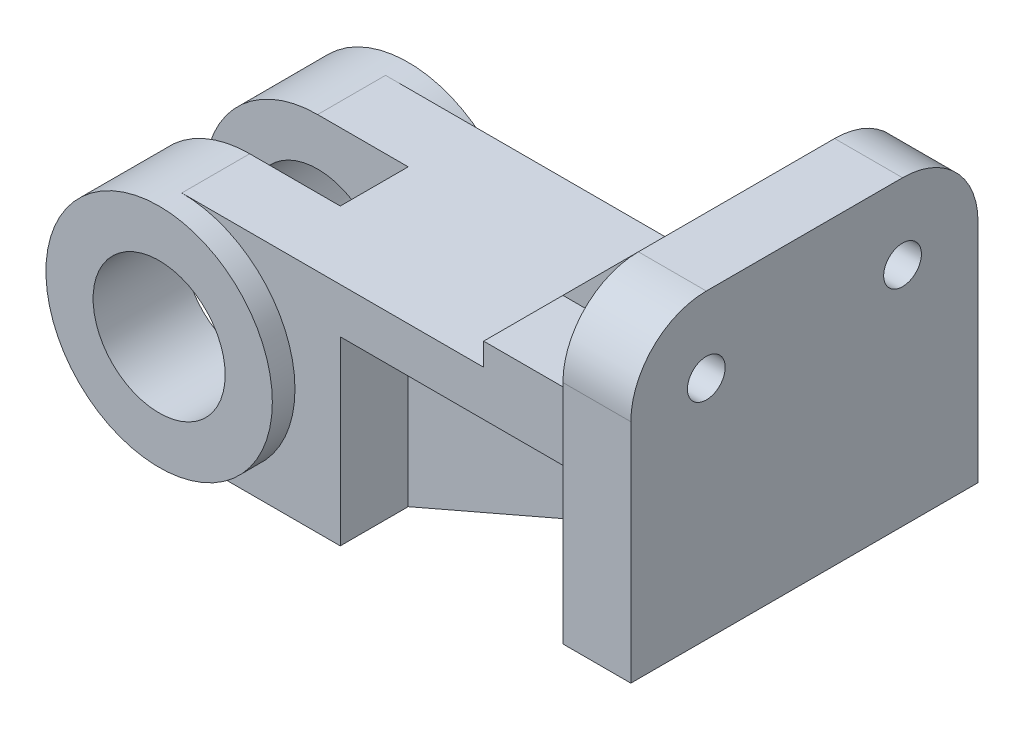
ISO-10303-21;
HEADER;
FILE_DESCRIPTION(('STEP AP214'),'2;1');
FILE_NAME('part.step','',(''),(''),'','','');
FILE_SCHEMA(('AUTOMOTIVE_DESIGN { 1 0 10303 214 1 1 1 1 }'));
ENDSEC;
DATA;
#1=APPLICATION_CONTEXT('core data for automotive mechanical design processes');
#2=APPLICATION_PROTOCOL_DEFINITION('international standard','automotive_design',2000,#1);
#3=PRODUCT_CONTEXT('',#1,'mechanical');
#4=PRODUCT('Part','Part','',(#3));
#5=PRODUCT_RELATED_PRODUCT_CATEGORY('part','',(#4));
#6=PRODUCT_DEFINITION_FORMATION('','',#4);
#7=PRODUCT_DEFINITION_CONTEXT('part definition',#1,'design');
#8=PRODUCT_DEFINITION('design','',#6,#7);
#9=PRODUCT_DEFINITION_SHAPE('','',#8);
#10=(LENGTH_UNIT() NAMED_UNIT(*) SI_UNIT(.MILLI.,.METRE.));
#11=(NAMED_UNIT(*) PLANE_ANGLE_UNIT() SI_UNIT($,.RADIAN.));
#12=(NAMED_UNIT(*) SI_UNIT($,.STERADIAN.) SOLID_ANGLE_UNIT());
#13=UNCERTAINTY_MEASURE_WITH_UNIT(LENGTH_MEASURE(1.E-05),#10,'distance_accuracy_value','');
#14=(GEOMETRIC_REPRESENTATION_CONTEXT(3) GLOBAL_UNCERTAINTY_ASSIGNED_CONTEXT((#13)) GLOBAL_UNIT_ASSIGNED_CONTEXT((#10,
#11,#12)) REPRESENTATION_CONTEXT('',''));
#15=CARTESIAN_POINT('',(0.,0.,0.));
#16=DIRECTION('',(0.,0.,1.));
#17=DIRECTION('',(1.,0.,0.));
#18=AXIS2_PLACEMENT_3D('',#15,#16,#17);
#19=CARTESIAN_POINT('',(0.,0.,33.));
#20=DIRECTION('',(0.,0.,-1.));
#21=DIRECTION('',(-1.,0.,0.));
#22=AXIS2_PLACEMENT_3D('',#19,#20,#21);
#23=CYLINDRICAL_SURFACE('',#22,30.);
#24=CARTESIAN_POINT('',(0.,0.,-33.));
#25=DIRECTION('',(0.,0.,1.));
#26=DIRECTION('',(1.,0.,0.));
#27=AXIS2_PLACEMENT_3D('',#24,#25,#26);
#28=CIRCLE('',#27,30.);
#29=CARTESIAN_POINT('',(30.,0.,-33.));
#30=VERTEX_POINT('',#29);
#31=EDGE_CURVE('E454',#30,#30,#28,.T.);
#32=ORIENTED_EDGE('',*,*,#31,.T.);
#33=EDGE_LOOP('',(#32));
#34=FACE_BOUND('',#33,.T.);
#35=DIRECTION('',(0.,0.,-1.));
#36=VECTOR('',#35,1.);
#37=CARTESIAN_POINT('',(0.,-30.,27.));
#38=LINE('',#37,#36);
#39=CARTESIAN_POINT('',(0.,-30.,-9.));
#40=VERTEX_POINT('',#39);
#41=CARTESIAN_POINT('',(0.,-30.,-27.));
#42=VERTEX_POINT('',#41);
#43=EDGE_CURVE('E446',#40,#42,#38,.T.);
#44=ORIENTED_EDGE('',*,*,#43,.F.);
#45=CARTESIAN_POINT('',(0.,0.,-9.));
#46=DIRECTION('',(0.,0.,-1.));
#47=DIRECTION('',(-1.,0.,0.));
#48=AXIS2_PLACEMENT_3D('',#45,#46,#47);
#49=CIRCLE('',#48,30.);
#50=CARTESIAN_POINT('',(0.,30.,-9.));
#51=VERTEX_POINT('',#50);
#52=EDGE_CURVE('E256',#40,#51,#49,.T.);
#53=ORIENTED_EDGE('',*,*,#52,.T.);
#54=DIRECTION('',(0.,0.,-1.));
#55=VECTOR('',#54,1.);
#56=CARTESIAN_POINT('',(0.,30.,27.));
#57=LINE('',#56,#55);
#58=CARTESIAN_POINT('',(0.,30.,-27.));
#59=VERTEX_POINT('',#58);
#60=EDGE_CURVE('E388',#51,#59,#57,.T.);
#61=ORIENTED_EDGE('',*,*,#60,.T.);
#62=CARTESIAN_POINT('',(0.,0.,-27.));
#63=DIRECTION('',(0.,0.,-1.));
#64=DIRECTION('',(1.,0.,0.));
#65=AXIS2_PLACEMENT_3D('',#62,#63,#64);
#66=CIRCLE('',#65,30.);
#67=EDGE_CURVE('E365',#59,#42,#66,.T.);
#68=ORIENTED_EDGE('',*,*,#67,.T.);
#69=EDGE_LOOP('',(#44,#53,#61,#68));
#70=FACE_BOUND('',#69,.T.);
#71=ADVANCED_FACE('F44',(#34,#70),#23,.T.);
#72=CARTESIAN_POINT('',(0.,0.,33.));
#73=DIRECTION('',(0.,0.,-1.));
#74=DIRECTION('',(-1.,0.,0.));
#75=AXIS2_PLACEMENT_3D('',#72,#73,#74);
#76=CYLINDRICAL_SURFACE('',#75,17.5);
#77=CARTESIAN_POINT('',(0.,0.,-9.));
#78=DIRECTION('',(0.,0.,-1.));
#79=DIRECTION('',(-1.,0.,0.));
#80=AXIS2_PLACEMENT_3D('',#77,#78,#79);
#81=CIRCLE('',#80,17.5);
#82=CARTESIAN_POINT('',(-17.5,0.,-9.));
#83=VERTEX_POINT('',#82);
#84=EDGE_CURVE('E254',#83,#83,#81,.T.);
#85=ORIENTED_EDGE('',*,*,#84,.F.);
#86=EDGE_LOOP('',(#85));
#87=FACE_BOUND('',#86,.T.);
#88=CARTESIAN_POINT('',(0.,0.,-33.));
#89=DIRECTION('',(0.,0.,1.));
#90=DIRECTION('',(1.,0.,0.));
#91=AXIS2_PLACEMENT_3D('',#88,#89,#90);
#92=CIRCLE('',#91,17.5);
#93=CARTESIAN_POINT('',(17.5,0.,-33.));
#94=VERTEX_POINT('',#93);
#95=EDGE_CURVE('E447',#94,#94,#92,.T.);
#96=ORIENTED_EDGE('',*,*,#95,.F.);
#97=EDGE_LOOP('',(#96));
#98=FACE_BOUND('',#97,.T.);
#99=ADVANCED_FACE('F469',(#87,#98),#76,.F.);
#100=CARTESIAN_POINT('',(120.,36.,27.));
#101=DIRECTION('',(0.,-1.,0.));
#102=DIRECTION('',(1.,0.,0.));
#103=AXIS2_PLACEMENT_3D('',#100,#101,#102);
#104=PLANE('',#103);
#105=DIRECTION('',(-1.,0.,0.));
#106=VECTOR('',#105,1.);
#107=CARTESIAN_POINT('',(120.,36.,-6.));
#108=LINE('',#107,#106);
#109=CARTESIAN_POINT('',(120.,36.,-6.));
#110=VERTEX_POINT('',#109);
#111=CARTESIAN_POINT('',(80.,36.,-6.));
#112=VERTEX_POINT('',#111);
#113=EDGE_CURVE('E268',#110,#112,#108,.T.);
#114=ORIENTED_EDGE('',*,*,#113,.F.);
#115=DIRECTION('',(0.,0.,-1.));
#116=VECTOR('',#115,1.);
#117=CARTESIAN_POINT('',(120.,36.,27.));
#118=LINE('',#117,#116);
#119=CARTESIAN_POINT('',(120.,36.,-27.));
#120=VERTEX_POINT('',#119);
#121=EDGE_CURVE('E428',#110,#120,#118,.T.);
#122=ORIENTED_EDGE('',*,*,#121,.T.);
#123=DIRECTION('',(-1.,0.,0.));
#124=VECTOR('',#123,1.);
#125=CARTESIAN_POINT('',(120.,36.,-27.));
#126=LINE('',#125,#124);
#127=CARTESIAN_POINT('',(80.,36.,-27.));
#128=VERTEX_POINT('',#127);
#129=EDGE_CURVE('E412',#120,#128,#126,.T.);
#130=ORIENTED_EDGE('',*,*,#129,.T.);
#131=DIRECTION('',(0.,0.,-1.));
#132=VECTOR('',#131,1.);
#133=CARTESIAN_POINT('',(80.,36.,27.));
#134=LINE('',#133,#132);
#135=EDGE_CURVE('E424',#112,#128,#134,.T.);
#136=ORIENTED_EDGE('',*,*,#135,.F.);
#137=EDGE_LOOP('',(#114,#122,#130,#136));
#138=FACE_BOUND('',#137,.T.);
#139=ADVANCED_FACE('F473',(#138),#104,.F.);
#140=CARTESIAN_POINT('',(120.,56.,26.));
#141=DIRECTION('',(-1.,0.,0.));
#142=DIRECTION('',(0.,0.,1.));
#143=AXIS2_PLACEMENT_3D('',#140,#141,#142);
#144=PLANE('',#143);
#145=CARTESIAN_POINT('',(120.,56.,-26.));
#146=DIRECTION('',(1.,0.,0.));
#147=DIRECTION('',(0.,0.,-1.));
#148=AXIS2_PLACEMENT_3D('',#145,#146,#147);
#149=CIRCLE('',#148,5.);
#150=CARTESIAN_POINT('',(120.,56.,-31.));
#151=VERTEX_POINT('',#150);
#152=EDGE_CURVE('E280',#151,#151,#149,.T.);
#153=ORIENTED_EDGE('',*,*,#152,.T.);
#154=EDGE_LOOP('',(#153));
#155=FACE_BOUND('',#154,.T.);
#156=ORIENTED_EDGE('',*,*,#121,.F.);
#157=DIRECTION('',(0.,1.,0.));
#158=VECTOR('',#157,1.);
#159=CARTESIAN_POINT('',(120.,56.,-6.));
#160=LINE('',#159,#158);
#161=CARTESIAN_POINT('',(120.,76.,-6.));
#162=VERTEX_POINT('',#161);
#163=EDGE_CURVE('E263',#110,#162,#160,.T.);
#164=ORIENTED_EDGE('',*,*,#163,.T.);
#165=DIRECTION('',(0.,0.,1.));
#166=VECTOR('',#165,1.);
#167=CARTESIAN_POINT('',(120.,76.,26.));
#168=LINE('',#167,#166);
#169=CARTESIAN_POINT('',(120.,76.,-26.));
#170=VERTEX_POINT('',#169);
#171=EDGE_CURVE('E316',#170,#162,#168,.T.);
#172=ORIENTED_EDGE('',*,*,#171,.F.);
#173=CARTESIAN_POINT('',(120.,56.,-26.));
#174=DIRECTION('',(1.,0.,0.));
#175=DIRECTION('',(0.,0.,1.));
#176=AXIS2_PLACEMENT_3D('',#173,#174,#175);
#177=CIRCLE('',#176,20.);
#178=CARTESIAN_POINT('',(120.,56.,-46.));
#179=VERTEX_POINT('',#178);
#180=EDGE_CURVE('E311',#179,#170,#177,.T.);
#181=ORIENTED_EDGE('',*,*,#180,.F.);
#182=DIRECTION('',(0.,1.,0.));
#183=VECTOR('',#182,1.);
#184=CARTESIAN_POINT('',(120.,-4.,-46.));
#185=LINE('',#184,#183);
#186=CARTESIAN_POINT('',(120.,-4.,-46.));
#187=VERTEX_POINT('',#186);
#188=EDGE_CURVE('E313',#187,#179,#185,.T.);
#189=ORIENTED_EDGE('',*,*,#188,.F.);
#190=DIRECTION('',(0.,0.,-1.));
#191=VECTOR('',#190,1.);
#192=CARTESIAN_POINT('',(120.,-4.,46.));
#193=LINE('',#192,#191);
#194=CARTESIAN_POINT('',(120.,-4.,-27.));
#195=VERTEX_POINT('',#194);
#196=EDGE_CURVE('E307',#195,#187,#193,.T.);
#197=ORIENTED_EDGE('',*,*,#196,.F.);
#198=DIRECTION('',(0.,1.,0.));
#199=VECTOR('',#198,1.);
#200=CARTESIAN_POINT('',(120.,36.,-27.));
#201=LINE('',#200,#199);
#202=EDGE_CURVE('E406',#195,#120,#201,.T.);
#203=ORIENTED_EDGE('',*,*,#202,.T.);
#204=EDGE_LOOP('',(#156,#164,#172,#181,#189,#197,#203));
#205=FACE_BOUND('',#204,.T.);
#206=ADVANCED_FACE('F479',(#155,#205),#144,.T.);
#207=CARTESIAN_POINT('',(42.,18.,27.));
#208=DIRECTION('',(-1.,0.,0.));
#209=DIRECTION('',(0.,-1.,0.));
#210=AXIS2_PLACEMENT_3D('',#207,#208,#209);
#211=PLANE('',#210);
#212=DIRECTION('',(0.,1.,0.));
#213=VECTOR('',#212,1.);
#214=CARTESIAN_POINT('',(42.,18.,-9.00000000000001));
#215=LINE('',#214,#213);
#216=CARTESIAN_POINT('',(42.,-30.,-9.));
#217=VERTEX_POINT('',#216);
#218=CARTESIAN_POINT('',(42.,18.,-9.00000000000001));
#219=VERTEX_POINT('',#218);
#220=EDGE_CURVE('E345',#217,#219,#215,.T.);
#221=ORIENTED_EDGE('',*,*,#220,.F.);
#222=DIRECTION('',(0.,0.,-1.));
#223=VECTOR('',#222,1.);
#224=CARTESIAN_POINT('',(42.,-30.,27.));
#225=LINE('',#224,#223);
#226=CARTESIAN_POINT('',(42.,-30.,-27.));
#227=VERTEX_POINT('',#226);
#228=EDGE_CURVE('E441',#217,#227,#225,.T.);
#229=ORIENTED_EDGE('',*,*,#228,.T.);
#230=DIRECTION('',(0.,1.,0.));
#231=VECTOR('',#230,1.);
#232=CARTESIAN_POINT('',(42.,18.,-27.));
#233=LINE('',#232,#231);
#234=CARTESIAN_POINT('',(42.,18.,-27.));
#235=VERTEX_POINT('',#234);
#236=EDGE_CURVE('E397',#227,#235,#233,.T.);
#237=ORIENTED_EDGE('',*,*,#236,.T.);
#238=DIRECTION('',(0.,0.,-1.));
#239=VECTOR('',#238,1.);
#240=CARTESIAN_POINT('',(42.,18.,27.));
#241=LINE('',#240,#239);
#242=EDGE_CURVE('E439',#219,#235,#241,.T.);
#243=ORIENTED_EDGE('',*,*,#242,.F.);
#244=EDGE_LOOP('',(#221,#229,#237,#243));
#245=FACE_BOUND('',#244,.T.);
#246=ADVANCED_FACE('F513',(#245),#211,.F.);
#247=CARTESIAN_POINT('',(42.,18.,27.));
#248=DIRECTION('',(0.,1.,0.));
#249=DIRECTION('',(0.,0.,1.));
#250=AXIS2_PLACEMENT_3D('',#247,#248,#249);
#251=PLANE('',#250);
#252=DIRECTION('',(1.,0.,0.));
#253=VECTOR('',#252,1.);
#254=CARTESIAN_POINT('',(42.,18.,-9.00000000000001));
#255=LINE('',#254,#253);
#256=CARTESIAN_POINT('',(102.,18.,-9.00000000000001));
#257=VERTEX_POINT('',#256);
#258=EDGE_CURVE('E347',#219,#257,#255,.T.);
#259=ORIENTED_EDGE('',*,*,#258,.F.);
#260=ORIENTED_EDGE('',*,*,#242,.T.);
#261=DIRECTION('',(1.,0.,0.));
#262=VECTOR('',#261,1.);
#263=CARTESIAN_POINT('',(42.,18.,-27.));
#264=LINE('',#263,#262);
#265=CARTESIAN_POINT('',(102.,18.,-27.));
#266=VERTEX_POINT('',#265);
#267=EDGE_CURVE('E399',#235,#266,#264,.T.);
#268=ORIENTED_EDGE('',*,*,#267,.T.);
#269=DIRECTION('',(0.,0.,-1.));
#270=VECTOR('',#269,1.);
#271=CARTESIAN_POINT('',(102.,18.,27.));
#272=LINE('',#271,#270);
#273=EDGE_CURVE('E436',#257,#266,#272,.T.);
#274=ORIENTED_EDGE('',*,*,#273,.F.);
#275=EDGE_LOOP('',(#259,#260,#268,#274));
#276=FACE_BOUND('',#275,.T.);
#277=ADVANCED_FACE('F502',(#276),#251,.F.);
#278=CARTESIAN_POINT('',(102.,-4.00000000000001,27.));
#279=DIRECTION('',(1.,0.,0.));
#280=DIRECTION('',(0.,0.,-1.));
#281=AXIS2_PLACEMENT_3D('',#278,#279,#280);
#282=PLANE('',#281);
#283=DIRECTION('',(0.,-1.,0.));
#284=VECTOR('',#283,1.);
#285=CARTESIAN_POINT('',(102.,-4.00000000000001,-9.00000000000001));
#286=LINE('',#285,#284);
#287=CARTESIAN_POINT('',(102.,-4.00000000000001,-9.00000000000001));
#288=VERTEX_POINT('',#287);
#289=EDGE_CURVE('E346',#257,#288,#286,.T.);
#290=ORIENTED_EDGE('',*,*,#289,.F.);
#291=ORIENTED_EDGE('',*,*,#273,.T.);
#292=DIRECTION('',(0.,-1.,0.));
#293=VECTOR('',#292,1.);
#294=CARTESIAN_POINT('',(102.,-4.00000000000001,-27.));
#295=LINE('',#294,#293);
#296=CARTESIAN_POINT('',(102.,-4.00000000000001,-27.));
#297=VERTEX_POINT('',#296);
#298=EDGE_CURVE('E405',#266,#297,#295,.T.);
#299=ORIENTED_EDGE('',*,*,#298,.T.);
#300=DIRECTION('',(0.,0.,-1.));
#301=VECTOR('',#300,1.);
#302=CARTESIAN_POINT('',(102.,-4.00000000000001,27.));
#303=LINE('',#302,#301);
#304=EDGE_CURVE('E435',#288,#297,#303,.T.);
#305=ORIENTED_EDGE('',*,*,#304,.F.);
#306=EDGE_LOOP('',(#290,#291,#299,#305));
#307=FACE_BOUND('',#306,.T.);
#308=ADVANCED_FACE('F498',(#307),#282,.F.);
#309=CARTESIAN_POINT('',(0.,0.,33.));
#310=DIRECTION('',(0.,0.,1.));
#311=DIRECTION('',(1.,0.,0.));
#312=AXIS2_PLACEMENT_3D('',#309,#310,#311);
#313=PLANE('',#312);
#314=CARTESIAN_POINT('',(0.,0.,33.));
#315=DIRECTION('',(0.,0.,1.));
#316=DIRECTION('',(1.,0.,0.));
#317=AXIS2_PLACEMENT_3D('',#314,#315,#316);
#318=CIRCLE('',#317,30.);
#319=CARTESIAN_POINT('',(30.,0.,33.));
#320=VERTEX_POINT('',#319);
#321=EDGE_CURVE('E52',#320,#320,#318,.T.);
#322=ORIENTED_EDGE('',*,*,#321,.T.);
#323=EDGE_LOOP('',(#322));
#324=FACE_BOUND('',#323,.T.);
#325=CARTESIAN_POINT('',(0.,0.,33.));
#326=DIRECTION('',(0.,0.,1.));
#327=DIRECTION('',(1.,0.,0.));
#328=AXIS2_PLACEMENT_3D('',#325,#326,#327);
#329=CIRCLE('',#328,17.5);
#330=CARTESIAN_POINT('',(17.5,0.,33.));
#331=VERTEX_POINT('',#330);
#332=EDGE_CURVE('E452',#331,#331,#329,.T.);
#333=ORIENTED_EDGE('',*,*,#332,.F.);
#334=EDGE_LOOP('',(#333));
#335=FACE_BOUND('',#334,.T.);
#336=ADVANCED_FACE('F467',(#324,#335),#313,.T.);
#337=CARTESIAN_POINT('',(0.,0.,-33.));
#338=DIRECTION('',(0.,0.,1.));
#339=DIRECTION('',(1.,0.,0.));
#340=AXIS2_PLACEMENT_3D('',#337,#338,#339);
#341=PLANE('',#340);
#342=ORIENTED_EDGE('',*,*,#31,.F.);
#343=EDGE_LOOP('',(#342));
#344=FACE_BOUND('',#343,.T.);
#345=ORIENTED_EDGE('',*,*,#95,.T.);
#346=EDGE_LOOP('',(#345));
#347=FACE_BOUND('',#346,.T.);
#348=ADVANCED_FACE('F461',(#344,#347),#341,.F.);
#349=CARTESIAN_POINT('',(0.,30.,27.));
#350=VERTEX_POINT('',#349);
#351=CARTESIAN_POINT('',(0.,30.,9.));
#352=VERTEX_POINT('',#351);
#353=EDGE_CURVE('E420',#350,#352,#57,.T.);
#354=ORIENTED_EDGE('',*,*,#353,.T.);
#355=CARTESIAN_POINT('',(0.,0.,9.));
#356=DIRECTION('',(0.,0.,1.));
#357=DIRECTION('',(1.,0.,0.));
#358=AXIS2_PLACEMENT_3D('',#355,#356,#357);
#359=CIRCLE('',#358,30.);
#360=CARTESIAN_POINT('',(0.,-30.,9.));
#361=VERTEX_POINT('',#360);
#362=EDGE_CURVE('E58',#352,#361,#359,.T.);
#363=ORIENTED_EDGE('',*,*,#362,.T.);
#364=CARTESIAN_POINT('',(0.,-30.,27.));
#365=VERTEX_POINT('',#364);
#366=EDGE_CURVE('E245',#365,#361,#38,.T.);
#367=ORIENTED_EDGE('',*,*,#366,.F.);
#368=CARTESIAN_POINT('',(0.,0.,27.));
#369=DIRECTION('',(0.,0.,-1.));
#370=DIRECTION('',(1.,0.,0.));
#371=AXIS2_PLACEMENT_3D('',#368,#369,#370);
#372=CIRCLE('',#371,30.);
#373=EDGE_CURVE('E364',#350,#365,#372,.T.);
#374=ORIENTED_EDGE('',*,*,#373,.F.);
#375=EDGE_LOOP('',(#354,#363,#367,#374));
#376=FACE_BOUND('',#375,.T.);
#377=ORIENTED_EDGE('',*,*,#321,.F.);
#378=EDGE_LOOP('',(#377));
#379=FACE_BOUND('',#378,.T.);
#380=ADVANCED_FACE('F50',(#376,#379),#23,.T.);
#381=CARTESIAN_POINT('',(0.,0.,9.));
#382=DIRECTION('',(0.,0.,1.));
#383=DIRECTION('',(1.,0.,0.));
#384=AXIS2_PLACEMENT_3D('',#381,#382,#383);
#385=CIRCLE('',#384,17.5);
#386=CARTESIAN_POINT('',(17.5,0.,9.));
#387=VERTEX_POINT('',#386);
#388=EDGE_CURVE('E246',#387,#387,#385,.T.);
#389=ORIENTED_EDGE('',*,*,#388,.F.);
#390=EDGE_LOOP('',(#389));
#391=FACE_BOUND('',#390,.T.);
#392=ORIENTED_EDGE('',*,*,#332,.T.);
#393=EDGE_LOOP('',(#392));
#394=FACE_BOUND('',#393,.T.);
#395=ADVANCED_FACE('F475',(#391,#394),#76,.F.);
#396=CARTESIAN_POINT('',(0.,-30.,27.));
#397=DIRECTION('',(0.,1.,0.));
#398=DIRECTION('',(0.,0.,1.));
#399=AXIS2_PLACEMENT_3D('',#396,#397,#398);
#400=PLANE('',#399);
#401=DIRECTION('',(0.,0.,-1.));
#402=VECTOR('',#401,1.);
#403=CARTESIAN_POINT('',(24.,-30.,-9.));
#404=LINE('',#403,#402);
#405=CARTESIAN_POINT('',(24.,-30.,9.));
#406=VERTEX_POINT('',#405);
#407=CARTESIAN_POINT('',(24.,-30.,-9.));
#408=VERTEX_POINT('',#407);
#409=EDGE_CURVE('E233',#406,#408,#404,.T.);
#410=ORIENTED_EDGE('',*,*,#409,.T.);
#411=DIRECTION('',(-1.,0.,0.));
#412=VECTOR('',#411,1.);
#413=CARTESIAN_POINT('',(-33.6386919250714,-30.,-9.));
#414=LINE('',#413,#412);
#415=EDGE_CURVE('E227',#408,#40,#414,.T.);
#416=ORIENTED_EDGE('',*,*,#415,.T.);
#417=ORIENTED_EDGE('',*,*,#43,.T.);
#418=DIRECTION('',(1.,0.,0.));
#419=VECTOR('',#418,1.);
#420=CARTESIAN_POINT('',(0.,-30.,-27.));
#421=LINE('',#420,#419);
#422=EDGE_CURVE('E391',#42,#227,#421,.T.);
#423=ORIENTED_EDGE('',*,*,#422,.T.);
#424=ORIENTED_EDGE('',*,*,#228,.F.);
#425=DIRECTION('',(0.,0.,1.));
#426=VECTOR('',#425,1.);
#427=CARTESIAN_POINT('',(42.,-30.,27.));
#428=LINE('',#427,#426);
#429=CARTESIAN_POINT('',(42.,-30.,9.));
#430=VERTEX_POINT('',#429);
#431=EDGE_CURVE('E362',#217,#430,#428,.T.);
#432=ORIENTED_EDGE('',*,*,#431,.T.);
#433=CARTESIAN_POINT('',(42.,-30.,27.));
#434=VERTEX_POINT('',#433);
#435=EDGE_CURVE('E443',#434,#430,#225,.T.);
#436=ORIENTED_EDGE('',*,*,#435,.F.);
#437=DIRECTION('',(1.,0.,0.));
#438=VECTOR('',#437,1.);
#439=CARTESIAN_POINT('',(0.,-30.,27.));
#440=LINE('',#439,#438);
#441=EDGE_CURVE('E366',#365,#434,#440,.T.);
#442=ORIENTED_EDGE('',*,*,#441,.F.);
#443=ORIENTED_EDGE('',*,*,#366,.T.);
#444=DIRECTION('',(1.,0.,0.));
#445=VECTOR('',#444,1.);
#446=CARTESIAN_POINT('',(24.,-30.,9.));
#447=LINE('',#446,#445);
#448=EDGE_CURVE('E223',#361,#406,#447,.T.);
#449=ORIENTED_EDGE('',*,*,#448,.T.);
#450=EDGE_LOOP('',(#410,#416,#417,#423,#424,#432,#436,#442,#443,#449));
#451=FACE_BOUND('',#450,.T.);
#452=ADVANCED_FACE('F238',(#451),#400,.F.);
#453=ORIENTED_EDGE('',*,*,#435,.T.);
#454=DIRECTION('',(0.,1.,0.));
#455=VECTOR('',#454,1.);
#456=CARTESIAN_POINT('',(42.,18.,9.));
#457=LINE('',#456,#455);
#458=CARTESIAN_POINT('',(42.,18.,9.));
#459=VERTEX_POINT('',#458);
#460=EDGE_CURVE('E353',#430,#459,#457,.T.);
#461=ORIENTED_EDGE('',*,*,#460,.T.);
#462=CARTESIAN_POINT('',(42.,18.,27.));
#463=VERTEX_POINT('',#462);
#464=EDGE_CURVE('E442',#463,#459,#241,.T.);
#465=ORIENTED_EDGE('',*,*,#464,.F.);
#466=DIRECTION('',(0.,1.,0.));
#467=VECTOR('',#466,1.);
#468=CARTESIAN_POINT('',(42.,18.,27.));
#469=LINE('',#468,#467);
#470=EDGE_CURVE('E371',#434,#463,#469,.T.);
#471=ORIENTED_EDGE('',*,*,#470,.F.);
#472=EDGE_LOOP('',(#453,#461,#465,#471));
#473=FACE_BOUND('',#472,.T.);
#474=ADVANCED_FACE('F495',(#473),#211,.F.);
#475=ORIENTED_EDGE('',*,*,#464,.T.);
#476=DIRECTION('',(1.,0.,0.));
#477=VECTOR('',#476,1.);
#478=CARTESIAN_POINT('',(42.,18.,9.));
#479=LINE('',#478,#477);
#480=CARTESIAN_POINT('',(102.,18.,9.));
#481=VERTEX_POINT('',#480);
#482=EDGE_CURVE('E354',#459,#481,#479,.T.);
#483=ORIENTED_EDGE('',*,*,#482,.T.);
#484=CARTESIAN_POINT('',(102.,18.,27.));
#485=VERTEX_POINT('',#484);
#486=EDGE_CURVE('E440',#485,#481,#272,.T.);
#487=ORIENTED_EDGE('',*,*,#486,.F.);
#488=DIRECTION('',(1.,0.,0.));
#489=VECTOR('',#488,1.);
#490=CARTESIAN_POINT('',(42.,18.,27.));
#491=LINE('',#490,#489);
#492=EDGE_CURVE('E373',#463,#485,#491,.T.);
#493=ORIENTED_EDGE('',*,*,#492,.F.);
#494=EDGE_LOOP('',(#475,#483,#487,#493));
#495=FACE_BOUND('',#494,.T.);
#496=ADVANCED_FACE('F516',(#495),#251,.F.);
#497=ORIENTED_EDGE('',*,*,#486,.T.);
#498=DIRECTION('',(0.,-1.,0.));
#499=VECTOR('',#498,1.);
#500=CARTESIAN_POINT('',(102.,-4.00000000000001,9.));
#501=LINE('',#500,#499);
#502=CARTESIAN_POINT('',(102.,-4.00000000000002,9.));
#503=VERTEX_POINT('',#502);
#504=EDGE_CURVE('E360',#481,#503,#501,.T.);
#505=ORIENTED_EDGE('',*,*,#504,.T.);
#506=CARTESIAN_POINT('',(102.,-4.00000000000001,27.));
#507=VERTEX_POINT('',#506);
#508=EDGE_CURVE('E433',#507,#503,#303,.T.);
#509=ORIENTED_EDGE('',*,*,#508,.F.);
#510=DIRECTION('',(0.,-1.,0.));
#511=VECTOR('',#510,1.);
#512=CARTESIAN_POINT('',(102.,-4.00000000000001,27.));
#513=LINE('',#512,#511);
#514=EDGE_CURVE('E374',#485,#507,#513,.T.);
#515=ORIENTED_EDGE('',*,*,#514,.F.);
#516=EDGE_LOOP('',(#497,#505,#509,#515));
#517=FACE_BOUND('',#516,.T.);
#518=ADVANCED_FACE('F508',(#517),#282,.F.);
#519=CARTESIAN_POINT('',(120.,-4.,27.));
#520=DIRECTION('',(0.,1.,0.));
#521=DIRECTION('',(-1.,0.,0.));
#522=AXIS2_PLACEMENT_3D('',#519,#520,#521);
#523=PLANE('',#522);
#524=DIRECTION('',(0.,0.,-1.));
#525=VECTOR('',#524,1.);
#526=CARTESIAN_POINT('',(102.,-4.00000000000001,27.));
#527=LINE('',#526,#525);
#528=EDGE_CURVE('E356',#503,#288,#527,.T.);
#529=ORIENTED_EDGE('',*,*,#528,.T.);
#530=ORIENTED_EDGE('',*,*,#304,.T.);
#531=DIRECTION('',(1.,0.,0.));
#532=VECTOR('',#531,1.);
#533=CARTESIAN_POINT('',(120.,-4.,-27.));
#534=LINE('',#533,#532);
#535=EDGE_CURVE('E403',#297,#195,#534,.T.);
#536=ORIENTED_EDGE('',*,*,#535,.T.);
#537=ORIENTED_EDGE('',*,*,#196,.T.);
#538=DIRECTION('',(-1.,0.,0.));
#539=VECTOR('',#538,1.);
#540=CARTESIAN_POINT('',(138.,-4.,-46.));
#541=LINE('',#540,#539);
#542=CARTESIAN_POINT('',(138.,-4.,-46.));
#543=VERTEX_POINT('',#542);
#544=EDGE_CURVE('E335',#543,#187,#541,.T.);
#545=ORIENTED_EDGE('',*,*,#544,.F.);
#546=DIRECTION('',(0.,0.,-1.));
#547=VECTOR('',#546,1.);
#548=CARTESIAN_POINT('',(138.,-4.,46.));
#549=LINE('',#548,#547);
#550=CARTESIAN_POINT('',(138.,-4.,46.));
#551=VERTEX_POINT('',#550);
#552=EDGE_CURVE('E291',#551,#543,#549,.T.);
#553=ORIENTED_EDGE('',*,*,#552,.F.);
#554=DIRECTION('',(-1.,0.,0.));
#555=VECTOR('',#554,1.);
#556=CARTESIAN_POINT('',(138.,-4.,46.));
#557=LINE('',#556,#555);
#558=CARTESIAN_POINT('',(120.,-4.,46.));
#559=VERTEX_POINT('',#558);
#560=EDGE_CURVE('E333',#551,#559,#557,.T.);
#561=ORIENTED_EDGE('',*,*,#560,.T.);
#562=CARTESIAN_POINT('',(120.,-4.,27.));
#563=VERTEX_POINT('',#562);
#564=EDGE_CURVE('E306',#559,#563,#193,.T.);
#565=ORIENTED_EDGE('',*,*,#564,.T.);
#566=DIRECTION('',(1.,0.,0.));
#567=VECTOR('',#566,1.);
#568=CARTESIAN_POINT('',(120.,-4.,27.));
#569=LINE('',#568,#567);
#570=EDGE_CURVE('E380',#507,#563,#569,.T.);
#571=ORIENTED_EDGE('',*,*,#570,.F.);
#572=ORIENTED_EDGE('',*,*,#508,.T.);
#573=EDGE_LOOP('',(#529,#530,#536,#537,#545,#553,#561,#565,#571,#572));
#574=FACE_BOUND('',#573,.T.);
#575=ADVANCED_FACE('F525',(#574),#523,.F.);
#576=CARTESIAN_POINT('',(120.,36.,27.));
#577=VERTEX_POINT('',#576);
#578=CARTESIAN_POINT('',(120.,36.,6.));
#579=VERTEX_POINT('',#578);
#580=EDGE_CURVE('E427',#577,#579,#118,.T.);
#581=ORIENTED_EDGE('',*,*,#580,.T.);
#582=DIRECTION('',(-1.,0.,0.));
#583=VECTOR('',#582,1.);
#584=CARTESIAN_POINT('',(120.,36.,6.));
#585=LINE('',#584,#583);
#586=CARTESIAN_POINT('',(80.,36.,6.));
#587=VERTEX_POINT('',#586);
#588=EDGE_CURVE('E275',#579,#587,#585,.T.);
#589=ORIENTED_EDGE('',*,*,#588,.T.);
#590=CARTESIAN_POINT('',(80.,36.,27.));
#591=VERTEX_POINT('',#590);
#592=EDGE_CURVE('E422',#591,#587,#134,.T.);
#593=ORIENTED_EDGE('',*,*,#592,.F.);
#594=DIRECTION('',(-1.,0.,0.));
#595=VECTOR('',#594,1.);
#596=CARTESIAN_POINT('',(120.,36.,27.));
#597=LINE('',#596,#595);
#598=EDGE_CURVE('E382',#577,#591,#597,.T.);
#599=ORIENTED_EDGE('',*,*,#598,.F.);
#600=EDGE_LOOP('',(#581,#589,#593,#599));
#601=FACE_BOUND('',#600,.T.);
#602=ADVANCED_FACE('F485',(#601),#104,.F.);
#603=CARTESIAN_POINT('',(80.,36.,27.));
#604=DIRECTION('',(1.,0.,0.));
#605=DIRECTION('',(0.,0.,-1.));
#606=AXIS2_PLACEMENT_3D('',#603,#604,#605);
#607=PLANE('',#606);
#608=ORIENTED_EDGE('',*,*,#592,.T.);
#609=DIRECTION('',(0.,0.,-1.));
#610=VECTOR('',#609,1.);
#611=CARTESIAN_POINT('',(80.,36.,27.));
#612=LINE('',#611,#610);
#613=EDGE_CURVE('E274',#112,#587,#612,.F.);
#614=ORIENTED_EDGE('',*,*,#613,.F.);
#615=ORIENTED_EDGE('',*,*,#135,.T.);
#616=DIRECTION('',(0.,-1.,0.));
#617=VECTOR('',#616,1.);
#618=CARTESIAN_POINT('',(80.,36.,-27.));
#619=LINE('',#618,#617);
#620=CARTESIAN_POINT('',(80.,30.,-27.));
#621=VERTEX_POINT('',#620);
#622=EDGE_CURVE('E414',#128,#621,#619,.T.);
#623=ORIENTED_EDGE('',*,*,#622,.T.);
#624=DIRECTION('',(0.,0.,-1.));
#625=VECTOR('',#624,1.);
#626=CARTESIAN_POINT('',(80.,30.,27.));
#627=LINE('',#626,#625);
#628=CARTESIAN_POINT('',(80.,30.,27.));
#629=VERTEX_POINT('',#628);
#630=EDGE_CURVE('E425',#629,#621,#627,.T.);
#631=ORIENTED_EDGE('',*,*,#630,.F.);
#632=DIRECTION('',(0.,-1.,0.));
#633=VECTOR('',#632,1.);
#634=CARTESIAN_POINT('',(80.,36.,27.));
#635=LINE('',#634,#633);
#636=EDGE_CURVE('E384',#591,#629,#635,.T.);
#637=ORIENTED_EDGE('',*,*,#636,.F.);
#638=EDGE_LOOP('',(#608,#614,#615,#623,#631,#637));
#639=FACE_BOUND('',#638,.T.);
#640=ADVANCED_FACE('F608',(#639),#607,.F.);
#641=CARTESIAN_POINT('',(0.,30.,27.));
#642=DIRECTION('',(0.,-1.,0.));
#643=DIRECTION('',(0.,0.,-1.));
#644=AXIS2_PLACEMENT_3D('',#641,#642,#643);
#645=PLANE('',#644);
#646=ORIENTED_EDGE('',*,*,#60,.F.);
#647=DIRECTION('',(-1.,0.,0.));
#648=VECTOR('',#647,1.);
#649=CARTESIAN_POINT('',(-33.6386919250714,30.,-9.));
#650=LINE('',#649,#648);
#651=CARTESIAN_POINT('',(24.,30.,-9.));
#652=VERTEX_POINT('',#651);
#653=EDGE_CURVE('E241',#652,#51,#650,.T.);
#654=ORIENTED_EDGE('',*,*,#653,.F.);
#655=DIRECTION('',(0.,0.,-1.));
#656=VECTOR('',#655,1.);
#657=CARTESIAN_POINT('',(24.,30.,-9.));
#658=LINE('',#657,#656);
#659=CARTESIAN_POINT('',(24.,30.,9.));
#660=VERTEX_POINT('',#659);
#661=EDGE_CURVE('E242',#660,#652,#658,.T.);
#662=ORIENTED_EDGE('',*,*,#661,.F.);
#663=DIRECTION('',(-1.,0.,0.));
#664=VECTOR('',#663,1.);
#665=CARTESIAN_POINT('',(0.,30.,9.));
#666=LINE('',#665,#664);
#667=EDGE_CURVE('E11',#660,#352,#666,.T.);
#668=ORIENTED_EDGE('',*,*,#667,.T.);
#669=ORIENTED_EDGE('',*,*,#353,.F.);
#670=DIRECTION('',(-1.,0.,0.));
#671=VECTOR('',#670,1.);
#672=CARTESIAN_POINT('',(45.6885172830265,30.,27.));
#673=LINE('',#672,#671);
#674=EDGE_CURVE('E390',#629,#350,#673,.T.);
#675=ORIENTED_EDGE('',*,*,#674,.F.);
#676=ORIENTED_EDGE('',*,*,#630,.T.);
#677=DIRECTION('',(-1.,0.,0.));
#678=VECTOR('',#677,1.);
#679=CARTESIAN_POINT('',(0.,30.,-27.));
#680=LINE('',#679,#678);
#681=EDGE_CURVE('E369',#621,#59,#680,.T.);
#682=ORIENTED_EDGE('',*,*,#681,.T.);
#683=EDGE_LOOP('',(#646,#654,#662,#668,#669,#675,#676,#682));
#684=FACE_BOUND('',#683,.T.);
#685=ADVANCED_FACE('F566',(#684),#645,.F.);
#686=CARTESIAN_POINT('',(0.,0.,27.));
#687=DIRECTION('',(0.,0.,1.));
#688=DIRECTION('',(1.,0.,0.));
#689=AXIS2_PLACEMENT_3D('',#686,#687,#688);
#690=PLANE('',#689);
#691=ORIENTED_EDGE('',*,*,#373,.T.);
#692=ORIENTED_EDGE('',*,*,#441,.T.);
#693=ORIENTED_EDGE('',*,*,#470,.T.);
#694=ORIENTED_EDGE('',*,*,#492,.T.);
#695=ORIENTED_EDGE('',*,*,#514,.T.);
#696=ORIENTED_EDGE('',*,*,#570,.T.);
#697=DIRECTION('',(0.,1.,0.));
#698=VECTOR('',#697,1.);
#699=CARTESIAN_POINT('',(120.,36.,27.));
#700=LINE('',#699,#698);
#701=EDGE_CURVE('E379',#563,#577,#700,.T.);
#702=ORIENTED_EDGE('',*,*,#701,.T.);
#703=ORIENTED_EDGE('',*,*,#598,.T.);
#704=ORIENTED_EDGE('',*,*,#636,.T.);
#705=ORIENTED_EDGE('',*,*,#674,.T.);
#706=EDGE_LOOP('',(#691,#692,#693,#694,#695,#696,#702,#703,#704,#705));
#707=FACE_BOUND('',#706,.T.);
#708=ADVANCED_FACE('F565',(#707),#690,.T.);
#709=CARTESIAN_POINT('',(0.,0.,-27.));
#710=DIRECTION('',(0.,0.,1.));
#711=DIRECTION('',(1.,0.,0.));
#712=AXIS2_PLACEMENT_3D('',#709,#710,#711);
#713=PLANE('',#712);
#714=ORIENTED_EDGE('',*,*,#67,.F.);
#715=ORIENTED_EDGE('',*,*,#681,.F.);
#716=ORIENTED_EDGE('',*,*,#622,.F.);
#717=ORIENTED_EDGE('',*,*,#129,.F.);
#718=ORIENTED_EDGE('',*,*,#202,.F.);
#719=ORIENTED_EDGE('',*,*,#535,.F.);
#720=ORIENTED_EDGE('',*,*,#298,.F.);
#721=ORIENTED_EDGE('',*,*,#267,.F.);
#722=ORIENTED_EDGE('',*,*,#236,.F.);
#723=ORIENTED_EDGE('',*,*,#422,.F.);
#724=EDGE_LOOP('',(#714,#715,#716,#717,#718,#719,#720,#721,#722,#723));
#725=FACE_BOUND('',#724,.T.);
#726=ADVANCED_FACE('F577',(#725),#713,.F.);
#727=CARTESIAN_POINT('',(42.,-30.,0.));
#728=DIRECTION('',(0.3976074376343,-0.917555625309924,0.));
#729=DIRECTION('',(0.917555625309924,0.3976074376343,0.));
#730=AXIS2_PLACEMENT_3D('',#727,#728,#729);
#731=PLANE('',#730);
#732=DIRECTION('',(0.917555625309924,0.3976074376343,0.));
#733=VECTOR('',#732,1.);
#734=CARTESIAN_POINT('',(42.,-30.,9.));
#735=LINE('',#734,#733);
#736=EDGE_CURVE('E339',#430,#503,#735,.T.);
#737=ORIENTED_EDGE('',*,*,#736,.F.);
#738=ORIENTED_EDGE('',*,*,#431,.F.);
#739=DIRECTION('',(0.917555625309924,0.3976074376343,0.));
#740=VECTOR('',#739,1.);
#741=CARTESIAN_POINT('',(42.,-30.,-9.));
#742=LINE('',#741,#740);
#743=EDGE_CURVE('E336',#217,#288,#742,.T.);
#744=ORIENTED_EDGE('',*,*,#743,.T.);
#745=ORIENTED_EDGE('',*,*,#528,.F.);
#746=EDGE_LOOP('',(#737,#738,#744,#745));
#747=FACE_BOUND('',#746,.T.);
#748=ADVANCED_FACE('F546',(#747),#731,.T.);
#749=CARTESIAN_POINT('',(45.,3.,9.));
#750=DIRECTION('',(0.,0.,1.));
#751=DIRECTION('',(1.,0.,0.));
#752=AXIS2_PLACEMENT_3D('',#749,#750,#751);
#753=PLANE('',#752);
#754=ORIENTED_EDGE('',*,*,#504,.F.);
#755=ORIENTED_EDGE('',*,*,#482,.F.);
#756=ORIENTED_EDGE('',*,*,#460,.F.);
#757=ORIENTED_EDGE('',*,*,#736,.T.);
#758=EDGE_LOOP('',(#754,#755,#756,#757));
#759=FACE_BOUND('',#758,.T.);
#760=ADVANCED_FACE('F538',(#759),#753,.T.);
#761=CARTESIAN_POINT('',(45.,3.,-9.));
#762=DIRECTION('',(0.,0.,1.));
#763=DIRECTION('',(1.,0.,0.));
#764=AXIS2_PLACEMENT_3D('',#761,#762,#763);
#765=PLANE('',#764);
#766=ORIENTED_EDGE('',*,*,#258,.T.);
#767=ORIENTED_EDGE('',*,*,#289,.T.);
#768=ORIENTED_EDGE('',*,*,#743,.F.);
#769=ORIENTED_EDGE('',*,*,#220,.T.);
#770=EDGE_LOOP('',(#766,#767,#768,#769));
#771=FACE_BOUND('',#770,.T.);
#772=ADVANCED_FACE('F548',(#771),#765,.F.);
#773=CARTESIAN_POINT('',(138.,56.,26.));
#774=DIRECTION('',(-1.,0.,0.));
#775=DIRECTION('',(0.,0.,1.));
#776=AXIS2_PLACEMENT_3D('',#773,#774,#775);
#777=PLANE('',#776);
#778=ORIENTED_EDGE('',*,*,#552,.T.);
#779=DIRECTION('',(0.,1.,0.));
#780=VECTOR('',#779,1.);
#781=CARTESIAN_POINT('',(138.,-4.,-46.));
#782=LINE('',#781,#780);
#783=CARTESIAN_POINT('',(138.,56.,-46.));
#784=VERTEX_POINT('',#783);
#785=EDGE_CURVE('E298',#543,#784,#782,.T.);
#786=ORIENTED_EDGE('',*,*,#785,.T.);
#787=CARTESIAN_POINT('',(138.,56.,-26.));
#788=DIRECTION('',(1.,0.,0.));
#789=DIRECTION('',(0.,0.,1.));
#790=AXIS2_PLACEMENT_3D('',#787,#788,#789);
#791=CIRCLE('',#790,20.);
#792=CARTESIAN_POINT('',(138.,76.,-26.));
#793=VERTEX_POINT('',#792);
#794=EDGE_CURVE('E296',#784,#793,#791,.T.);
#795=ORIENTED_EDGE('',*,*,#794,.T.);
#796=DIRECTION('',(0.,0.,1.));
#797=VECTOR('',#796,1.);
#798=CARTESIAN_POINT('',(138.,76.,26.));
#799=LINE('',#798,#797);
#800=CARTESIAN_POINT('',(138.,76.,26.));
#801=VERTEX_POINT('',#800);
#802=EDGE_CURVE('E297',#793,#801,#799,.T.);
#803=ORIENTED_EDGE('',*,*,#802,.T.);
#804=CARTESIAN_POINT('',(138.,56.,26.));
#805=DIRECTION('',(1.,0.,0.));
#806=DIRECTION('',(0.,0.,1.));
#807=AXIS2_PLACEMENT_3D('',#804,#805,#806);
#808=CIRCLE('',#807,20.);
#809=CARTESIAN_POINT('',(138.,56.,46.));
#810=VERTEX_POINT('',#809);
#811=EDGE_CURVE('E305',#801,#810,#808,.T.);
#812=ORIENTED_EDGE('',*,*,#811,.T.);
#813=DIRECTION('',(0.,-1.,0.));
#814=VECTOR('',#813,1.);
#815=CARTESIAN_POINT('',(138.,-4.,46.));
#816=LINE('',#815,#814);
#817=EDGE_CURVE('E286',#810,#551,#816,.T.);
#818=ORIENTED_EDGE('',*,*,#817,.T.);
#819=EDGE_LOOP('',(#778,#786,#795,#803,#812,#818));
#820=FACE_BOUND('',#819,.T.);
#821=CARTESIAN_POINT('',(138.,56.,26.));
#822=DIRECTION('',(1.,0.,0.));
#823=DIRECTION('',(0.,0.,-1.));
#824=AXIS2_PLACEMENT_3D('',#821,#822,#823);
#825=CIRCLE('',#824,5.);
#826=CARTESIAN_POINT('',(138.,56.,21.));
#827=VERTEX_POINT('',#826);
#828=EDGE_CURVE('E284',#827,#827,#825,.T.);
#829=ORIENTED_EDGE('',*,*,#828,.F.);
#830=EDGE_LOOP('',(#829));
#831=FACE_BOUND('',#830,.T.);
#832=CARTESIAN_POINT('',(138.,56.,-26.));
#833=DIRECTION('',(1.,0.,0.));
#834=DIRECTION('',(0.,0.,-1.));
#835=AXIS2_PLACEMENT_3D('',#832,#833,#834);
#836=CIRCLE('',#835,5.);
#837=CARTESIAN_POINT('',(138.,56.,-31.));
#838=VERTEX_POINT('',#837);
#839=EDGE_CURVE('E279',#838,#838,#836,.T.);
#840=ORIENTED_EDGE('',*,*,#839,.F.);
#841=EDGE_LOOP('',(#840));
#842=FACE_BOUND('',#841,.T.);
#843=ADVANCED_FACE('F587',(#820,#831,#842),#777,.F.);
#844=DIRECTION('',(0.,1.,0.));
#845=VECTOR('',#844,1.);
#846=CARTESIAN_POINT('',(120.,56.,6.));
#847=LINE('',#846,#845);
#848=CARTESIAN_POINT('',(120.,76.,6.));
#849=VERTEX_POINT('',#848);
#850=EDGE_CURVE('E269',#579,#849,#847,.T.);
#851=ORIENTED_EDGE('',*,*,#850,.F.);
#852=ORIENTED_EDGE('',*,*,#580,.F.);
#853=ORIENTED_EDGE('',*,*,#701,.F.);
#854=ORIENTED_EDGE('',*,*,#564,.F.);
#855=DIRECTION('',(0.,-1.,0.));
#856=VECTOR('',#855,1.);
#857=CARTESIAN_POINT('',(120.,-4.,46.));
#858=LINE('',#857,#856);
#859=CARTESIAN_POINT('',(120.,56.,46.));
#860=VERTEX_POINT('',#859);
#861=EDGE_CURVE('E290',#860,#559,#858,.T.);
#862=ORIENTED_EDGE('',*,*,#861,.F.);
#863=CARTESIAN_POINT('',(120.,56.,26.));
#864=DIRECTION('',(1.,0.,0.));
#865=DIRECTION('',(0.,0.,1.));
#866=AXIS2_PLACEMENT_3D('',#863,#864,#865);
#867=CIRCLE('',#866,20.);
#868=CARTESIAN_POINT('',(120.,76.,26.));
#869=VERTEX_POINT('',#868);
#870=EDGE_CURVE('E294',#869,#860,#867,.T.);
#871=ORIENTED_EDGE('',*,*,#870,.F.);
#872=EDGE_CURVE('E312',#849,#869,#168,.T.);
#873=ORIENTED_EDGE('',*,*,#872,.F.);
#874=EDGE_LOOP('',(#851,#852,#853,#854,#862,#871,#873));
#875=FACE_BOUND('',#874,.T.);
#876=CARTESIAN_POINT('',(120.,56.,26.));
#877=DIRECTION('',(1.,0.,0.));
#878=DIRECTION('',(0.,0.,-1.));
#879=AXIS2_PLACEMENT_3D('',#876,#877,#878);
#880=CIRCLE('',#879,5.);
#881=CARTESIAN_POINT('',(120.,56.,21.));
#882=VERTEX_POINT('',#881);
#883=EDGE_CURVE('E283',#882,#882,#880,.T.);
#884=ORIENTED_EDGE('',*,*,#883,.T.);
#885=EDGE_LOOP('',(#884));
#886=FACE_BOUND('',#885,.T.);
#887=ADVANCED_FACE('F605',(#875,#886),#144,.T.);
#888=CARTESIAN_POINT('',(138.,-4.,46.));
#889=DIRECTION('',(0.,0.,-1.));
#890=DIRECTION('',(-1.,0.,0.));
#891=AXIS2_PLACEMENT_3D('',#888,#889,#890);
#892=PLANE('',#891);
#893=ORIENTED_EDGE('',*,*,#861,.T.);
#894=ORIENTED_EDGE('',*,*,#560,.F.);
#895=ORIENTED_EDGE('',*,*,#817,.F.);
#896=DIRECTION('',(-1.,0.,0.));
#897=VECTOR('',#896,1.);
#898=CARTESIAN_POINT('',(138.,56.,46.));
#899=LINE('',#898,#897);
#900=EDGE_CURVE('E304',#810,#860,#899,.T.);
#901=ORIENTED_EDGE('',*,*,#900,.T.);
#902=EDGE_LOOP('',(#893,#894,#895,#901));
#903=FACE_BOUND('',#902,.T.);
#904=ADVANCED_FACE('F600',(#903),#892,.F.);
#905=CARTESIAN_POINT('',(138.,-4.,-46.));
#906=DIRECTION('',(0.,0.,1.));
#907=DIRECTION('',(1.,0.,0.));
#908=AXIS2_PLACEMENT_3D('',#905,#906,#907);
#909=PLANE('',#908);
#910=ORIENTED_EDGE('',*,*,#188,.T.);
#911=DIRECTION('',(-1.,0.,0.));
#912=VECTOR('',#911,1.);
#913=CARTESIAN_POINT('',(138.,56.,-46.));
#914=LINE('',#913,#912);
#915=EDGE_CURVE('E328',#784,#179,#914,.T.);
#916=ORIENTED_EDGE('',*,*,#915,.F.);
#917=ORIENTED_EDGE('',*,*,#785,.F.);
#918=ORIENTED_EDGE('',*,*,#544,.T.);
#919=EDGE_LOOP('',(#910,#916,#917,#918));
#920=FACE_BOUND('',#919,.T.);
#921=ADVANCED_FACE('F588',(#920),#909,.F.);
#922=CARTESIAN_POINT('',(138.,56.,-26.));
#923=DIRECTION('',(-1.,0.,0.));
#924=DIRECTION('',(0.,0.,1.));
#925=AXIS2_PLACEMENT_3D('',#922,#923,#924);
#926=CYLINDRICAL_SURFACE('',#925,20.);
#927=ORIENTED_EDGE('',*,*,#180,.T.);
#928=DIRECTION('',(-1.,0.,0.));
#929=VECTOR('',#928,1.);
#930=CARTESIAN_POINT('',(138.,76.,-26.));
#931=LINE('',#930,#929);
#932=EDGE_CURVE('E326',#793,#170,#931,.T.);
#933=ORIENTED_EDGE('',*,*,#932,.F.);
#934=ORIENTED_EDGE('',*,*,#794,.F.);
#935=ORIENTED_EDGE('',*,*,#915,.T.);
#936=EDGE_LOOP('',(#927,#933,#934,#935));
#937=FACE_BOUND('',#936,.T.);
#938=ADVANCED_FACE('F629',(#937),#926,.T.);
#939=CARTESIAN_POINT('',(138.,76.,26.));
#940=DIRECTION('',(0.,-1.,0.));
#941=DIRECTION('',(0.,0.,-1.));
#942=AXIS2_PLACEMENT_3D('',#939,#940,#941);
#943=PLANE('',#942);
#944=DIRECTION('',(-1.,0.,0.));
#945=VECTOR('',#944,1.);
#946=CARTESIAN_POINT('',(138.,76.,26.));
#947=LINE('',#946,#945);
#948=EDGE_CURVE('E323',#801,#869,#947,.T.);
#949=ORIENTED_EDGE('',*,*,#948,.F.);
#950=ORIENTED_EDGE('',*,*,#802,.F.);
#951=ORIENTED_EDGE('',*,*,#932,.T.);
#952=ORIENTED_EDGE('',*,*,#171,.T.);
#953=EDGE_CURVE('E317',#162,#849,#168,.T.);
#954=ORIENTED_EDGE('',*,*,#953,.T.);
#955=ORIENTED_EDGE('',*,*,#872,.T.);
#956=EDGE_LOOP('',(#949,#950,#951,#952,#954,#955));
#957=FACE_BOUND('',#956,.T.);
#958=ADVANCED_FACE('F625',(#957),#943,.F.);
#959=CARTESIAN_POINT('',(138.,56.,26.));
#960=DIRECTION('',(-1.,0.,0.));
#961=DIRECTION('',(0.,0.,1.));
#962=AXIS2_PLACEMENT_3D('',#959,#960,#961);
#963=CYLINDRICAL_SURFACE('',#962,20.);
#964=ORIENTED_EDGE('',*,*,#870,.T.);
#965=ORIENTED_EDGE('',*,*,#900,.F.);
#966=ORIENTED_EDGE('',*,*,#811,.F.);
#967=ORIENTED_EDGE('',*,*,#948,.T.);
#968=EDGE_LOOP('',(#964,#965,#966,#967));
#969=FACE_BOUND('',#968,.T.);
#970=ADVANCED_FACE('F628',(#969),#963,.T.);
#971=CARTESIAN_POINT('',(138.,56.,26.));
#972=DIRECTION('',(-1.,0.,0.));
#973=DIRECTION('',(0.,0.,1.));
#974=AXIS2_PLACEMENT_3D('',#971,#972,#973);
#975=CYLINDRICAL_SURFACE('',#974,5.);
#976=ORIENTED_EDGE('',*,*,#828,.T.);
#977=EDGE_LOOP('',(#976));
#978=FACE_BOUND('',#977,.T.);
#979=ORIENTED_EDGE('',*,*,#883,.F.);
#980=EDGE_LOOP('',(#979));
#981=FACE_BOUND('',#980,.T.);
#982=ADVANCED_FACE('F788',(#978,#981),#975,.F.);
#983=CARTESIAN_POINT('',(138.,56.,-26.));
#984=DIRECTION('',(-1.,0.,0.));
#985=DIRECTION('',(0.,0.,1.));
#986=AXIS2_PLACEMENT_3D('',#983,#984,#985);
#987=CYLINDRICAL_SURFACE('',#986,5.);
#988=ORIENTED_EDGE('',*,*,#839,.T.);
#989=EDGE_LOOP('',(#988));
#990=FACE_BOUND('',#989,.T.);
#991=ORIENTED_EDGE('',*,*,#152,.F.);
#992=EDGE_LOOP('',(#991));
#993=FACE_BOUND('',#992,.T.);
#994=ADVANCED_FACE('F702',(#990,#993),#987,.F.);
#995=CARTESIAN_POINT('',(80.,36.,0.));
#996=DIRECTION('',(0.707106781186548,-0.707106781186548,0.));
#997=DIRECTION('',(0.707106781186548,0.707106781186548,0.));
#998=AXIS2_PLACEMENT_3D('',#995,#996,#997);
#999=PLANE('',#998);
#1000=DIRECTION('',(0.707106781186548,0.707106781186548,0.));
#1001=VECTOR('',#1000,1.);
#1002=CARTESIAN_POINT('',(80.,36.,-6.));
#1003=LINE('',#1002,#1001);
#1004=EDGE_CURVE('E261',#112,#162,#1003,.T.);
#1005=ORIENTED_EDGE('',*,*,#1004,.F.);
#1006=ORIENTED_EDGE('',*,*,#613,.T.);
#1007=DIRECTION('',(0.707106781186548,0.707106781186548,0.));
#1008=VECTOR('',#1007,1.);
#1009=CARTESIAN_POINT('',(80.,36.,6.));
#1010=LINE('',#1009,#1008);
#1011=EDGE_CURVE('E70',#587,#849,#1010,.T.);
#1012=ORIENTED_EDGE('',*,*,#1011,.T.);
#1013=ORIENTED_EDGE('',*,*,#953,.F.);
#1014=EDGE_LOOP('',(#1005,#1006,#1012,#1013));
#1015=FACE_BOUND('',#1014,.T.);
#1016=ADVANCED_FACE('F618',(#1015),#999,.F.);
#1017=CARTESIAN_POINT('',(54.,23.,6.));
#1018=DIRECTION('',(0.,0.,1.));
#1019=DIRECTION('',(1.,0.,0.));
#1020=AXIS2_PLACEMENT_3D('',#1017,#1018,#1019);
#1021=PLANE('',#1020);
#1022=ORIENTED_EDGE('',*,*,#588,.F.);
#1023=ORIENTED_EDGE('',*,*,#850,.T.);
#1024=ORIENTED_EDGE('',*,*,#1011,.F.);
#1025=EDGE_LOOP('',(#1022,#1023,#1024));
#1026=FACE_BOUND('',#1025,.T.);
#1027=ADVANCED_FACE('F703',(#1026),#1021,.T.);
#1028=CARTESIAN_POINT('',(54.,23.,-6.));
#1029=DIRECTION('',(0.,0.,1.));
#1030=DIRECTION('',(1.,0.,0.));
#1031=AXIS2_PLACEMENT_3D('',#1028,#1029,#1030);
#1032=PLANE('',#1031);
#1033=ORIENTED_EDGE('',*,*,#163,.F.);
#1034=ORIENTED_EDGE('',*,*,#113,.T.);
#1035=ORIENTED_EDGE('',*,*,#1004,.T.);
#1036=EDGE_LOOP('',(#1033,#1034,#1035));
#1037=FACE_BOUND('',#1036,.T.);
#1038=ADVANCED_FACE('F620',(#1037),#1032,.F.);
#1039=CARTESIAN_POINT('',(-33.6386919250714,-30.,-9.));
#1040=DIRECTION('',(0.,0.,-1.));
#1041=DIRECTION('',(-1.,0.,0.));
#1042=AXIS2_PLACEMENT_3D('',#1039,#1040,#1041);
#1043=PLANE('',#1042);
#1044=ORIENTED_EDGE('',*,*,#84,.T.);
#1045=EDGE_LOOP('',(#1044));
#1046=FACE_BOUND('',#1045,.T.);
#1047=ORIENTED_EDGE('',*,*,#415,.F.);
#1048=DIRECTION('',(0.,1.,0.));
#1049=VECTOR('',#1048,1.);
#1050=CARTESIAN_POINT('',(24.,-30.,-9.));
#1051=LINE('',#1050,#1049);
#1052=EDGE_CURVE('E229',#408,#652,#1051,.T.);
#1053=ORIENTED_EDGE('',*,*,#1052,.T.);
#1054=ORIENTED_EDGE('',*,*,#653,.T.);
#1055=ORIENTED_EDGE('',*,*,#52,.F.);
#1056=EDGE_LOOP('',(#1047,#1053,#1054,#1055));
#1057=FACE_BOUND('',#1056,.T.);
#1058=ADVANCED_FACE('F573',(#1046,#1057),#1043,.F.);
#1059=CARTESIAN_POINT('',(24.,-30.,9.));
#1060=DIRECTION('',(0.,0.,1.));
#1061=DIRECTION('',(1.,0.,0.));
#1062=AXIS2_PLACEMENT_3D('',#1059,#1060,#1061);
#1063=PLANE('',#1062);
#1064=ORIENTED_EDGE('',*,*,#388,.T.);
#1065=EDGE_LOOP('',(#1064));
#1066=FACE_BOUND('',#1065,.T.);
#1067=ORIENTED_EDGE('',*,*,#667,.F.);
#1068=DIRECTION('',(0.,1.,0.));
#1069=VECTOR('',#1068,1.);
#1070=CARTESIAN_POINT('',(24.,-30.,9.));
#1071=LINE('',#1070,#1069);
#1072=EDGE_CURVE('E222',#406,#660,#1071,.T.);
#1073=ORIENTED_EDGE('',*,*,#1072,.F.);
#1074=ORIENTED_EDGE('',*,*,#448,.F.);
#1075=ORIENTED_EDGE('',*,*,#362,.F.);
#1076=EDGE_LOOP('',(#1067,#1073,#1074,#1075));
#1077=FACE_BOUND('',#1076,.T.);
#1078=ADVANCED_FACE('F224',(#1066,#1077),#1063,.F.);
#1079=CARTESIAN_POINT('',(24.,-30.,-9.));
#1080=DIRECTION('',(1.,0.,0.));
#1081=DIRECTION('',(0.,0.,-1.));
#1082=AXIS2_PLACEMENT_3D('',#1079,#1080,#1081);
#1083=PLANE('',#1082);
#1084=ORIENTED_EDGE('',*,*,#661,.T.);
#1085=ORIENTED_EDGE('',*,*,#1052,.F.);
#1086=ORIENTED_EDGE('',*,*,#409,.F.);
#1087=ORIENTED_EDGE('',*,*,#1072,.T.);
#1088=EDGE_LOOP('',(#1084,#1085,#1086,#1087));
#1089=FACE_BOUND('',#1088,.T.);
#1090=ADVANCED_FACE('F234',(#1089),#1083,.F.);
#1091=CLOSED_SHELL('',(#71,#99,#139,#206,#246,#277,#308,#336,#348,#380,#395,#452,#474,#496,#518,
#575,#602,#640,#685,#708,#726,#748,#760,#772,#843,#887,#904,#921,#938,#958,#970,#982,#994,#1016,
#1027,#1038,#1058,#1078,#1090));
#1092=MANIFOLD_SOLID_BREP('B2',#1091);
#1093=ADVANCED_BREP_SHAPE_REPRESENTATION('',(#18,#1092),#14);
#1094=SHAPE_DEFINITION_REPRESENTATION(#9,#1093);
ENDSEC;
END-ISO-10303-21;
